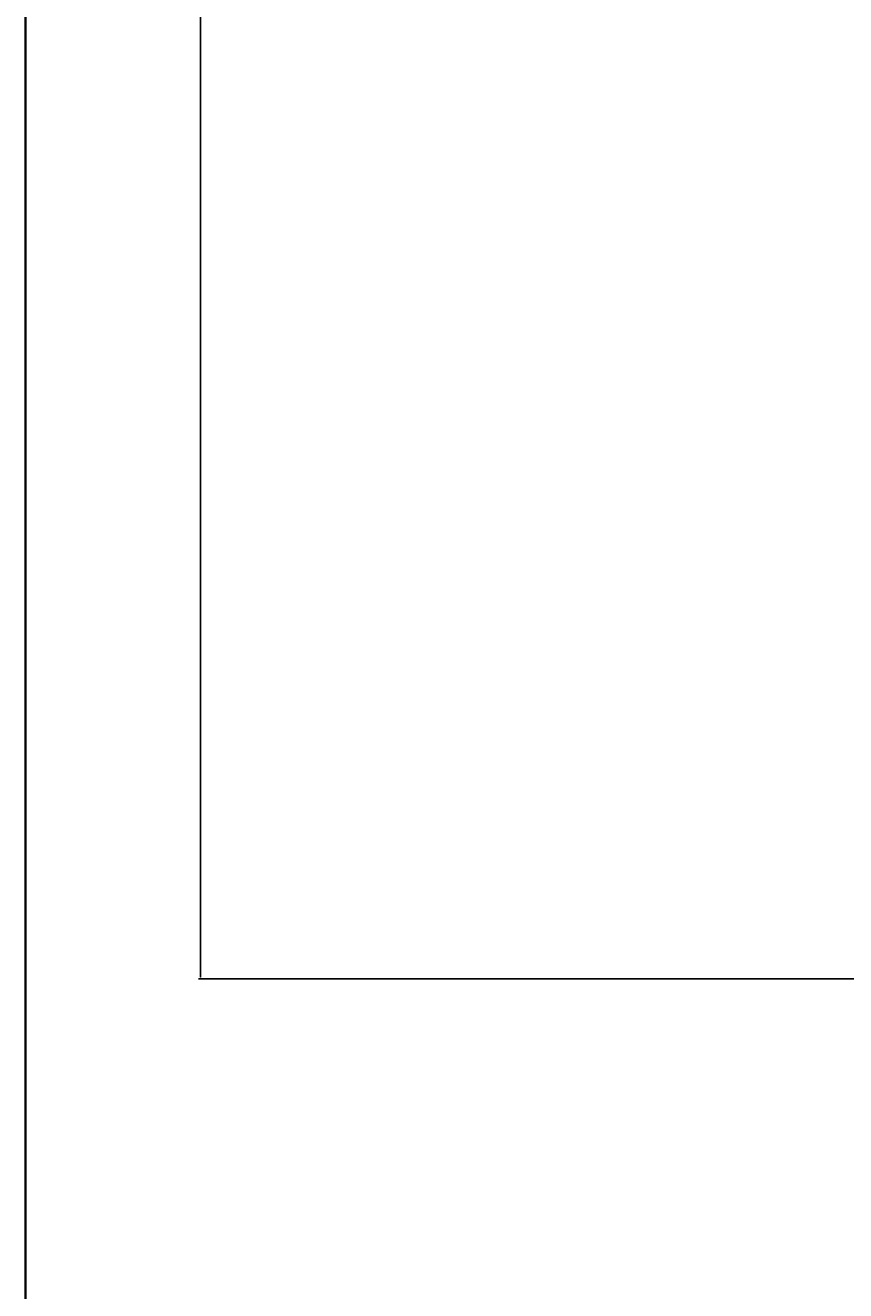
# Model space of a CAD drawing. Units: inches. Extents: x 1885 to 2748, y 783 to 2421.
# Tile 55 of 117: x 1885 to 1969, y 1850 to 1979. Entities that reach past the tile are written whole.
import ezdxf

# ---------------------------------------------------------------- set-up
doc = ezdxf.new("R2010")
doc.units = ezdxf.units.IN
doc.layers.add('A-ANNO-DIMS', color=2, linetype='Continuous', lineweight=18)
doc.layers.add('A-ANNO-TTLB', color=7, linetype='Continuous', lineweight=35)
doc.styles.get("Standard").update_dxf_attribs({"font": 'arial.ttf'})
doc.dimstyles.get("Standard").update_dxf_attribs({"dimtxt": 0.18, "dimasz": 0.18, "dimexe": 0.18, "dimexo": 0.0625, "dimgap": 0.09, "dimtad": 0, "dimtih": 1, "dimtoh": 1, "dimdec": 4, "dimzin": 0, "dimdsep": 46, "dimtxsty": 'Standard', "dimcen": 0.09, "dimadec": 0, "dimazin": 0, "dimtfac": 1, "dimtdec": 4, "dimtofl": 0, "dimtmove": 0, "dimatfit": 3, "dimfxl": 1, "dimtolj": 1, "dimtzin": 0, "dimarcsym": 0})

# ---------------------------------------------------------------- blocks, each defined once
blk = doc.blocks.new('*D48')
at = {"layer": 'A-ANNO-DIMS', "color": 0, "lineweight": -2, "transparency": 16777216}
for p, q in [((1980.71, 2348.01), (1902.84, 2348.01)), ((1903.02, 2347.83), (1903.02, 2114.94)), ((1903.02, 1881.69), (1903.02, 2114.57)), ((2016.71, 1881.51), (1902.84, 1881.51))]:
    blk.add_line(p, q, dxfattribs=at)
at = {"layer": 'A-ANNO-DIMS', "color": 0, "transparency": 16777216}
for points in [[(1902.99, 2347.83), (1903.05, 2347.83), (1903.02, 2348.01)], [(1902.99, 1881.69), (1903.05, 1881.69), (1903.02, 1881.51)]]:
    blk.add_solid(points, dxfattribs=at)
at = {"layer": 'Defpoints', "color": 0, "transparency": 16777216}
for p in [(1903.02, 2348.01), (1980.77, 2348.01), (2016.77, 1881.51)]:
    blk.add_point(p, dxfattribs=at)
at = {"layer": 'A-ANNO-DIMS', "color": 0, "transparency": 16777216, "insert": (1903.02, 2114.76), "char_height": 0.18, "attachment_point": 5}
blk.add_mtext('\\A1;466.5', dxfattribs=at)

msp = doc.modelspace()

# ---------------------------------------------------------------- linework, layer by layer
at = {"layer": 'A-ANNO-TTLB'}
msp.add_lwpolyline([(1885.16, 2409.17), (2748.2, 2409.17), (2748.2, 922.58), (1885.16, 922.58)], close=True, dxfattribs=at)

# ---------------------------------------------------------------- dimensions: what is measured, and where the dimension line sits
at = {"layer": 'A-ANNO-DIMS'}
dim = msp.add_linear_dim(base=(1903.02, 2348.01), p1=(2016.77, 1881.51), p2=(1980.77, 2348.01), angle=90, dimstyle='Standard', override={"dimdec": 1, "dimlfac": 1, "dimrnd": 0, "dimzin": 0, "dimdsep": 46, "dimlunit": 2}, dxfattribs=at)
dim.commit()
dim.dimension.update_dxf_attribs({"geometry": '*D48', "text_midpoint": (1903.02, 2114.76)})

doc.saveas('drawing.dxf')
